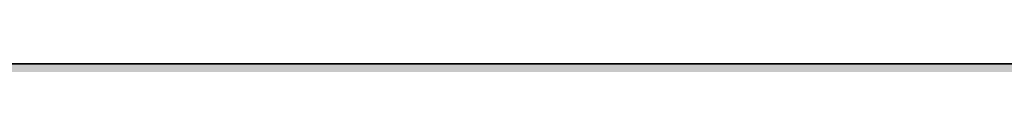
# Model space of a CAD drawing. Units: inches. Extents: x 2091 to 2899, y 967 to 2217.
# Tile 64 of 256: x 2212.2941 to 2212.646, y 1099.9191 to 1099.9191. Entities that reach past the tile are written whole.
import ezdxf

# ---------------------------------------------------------------- set-up
doc = ezdxf.new("R2010")
doc.units = ezdxf.units.IN
doc.layers.add('A-WALL-PATT', color=141, linetype='Continuous', lineweight=13, true_color=0xadddf7)
doc.layers.add('L-SITE-WALL', color=7, linetype='Continuous', lineweight=35)

msp = doc.modelspace()

# ---------------------------------------------------------------- hatches: boundary and pattern name
at = {"layer": 'A-WALL-PATT'}
h = msp.add_hatch(color=256, dxfattribs=at)
h.dxf.hatch_style = 1
h.paths.add_polyline_path([(2212.1436, 1941.41906), (2387.6436, 1941.41906), (2387.6436, 1824.41906), (2392.1436, 1824.41906), (2392.1436, 1941.41906), (2609.6436, 1941.41906), (2609.6436, 1825.91906), (2614.1436, 1825.91906), (2614.1436, 1941.41906), (2794.1436, 1941.41906), (2794.1436, 1928.76217), (2803.1436, 1928.76217), (2803.1436, 2050.91906), (2203.1436, 2050.91906), (2203.1436, 1900.75786), (2212.1436, 1900.75786)])
h.paths.add_polyline_path([(2212.1436, 1945.91906), (2212.1436, 2041.91906), (2794.1436, 2041.91906), (2794.1436, 1945.91906), (2402.24824, 1945.91906), (2401.10243, 1945.77583), (2398.70243, 1945.77583)], flags=16)
h.paths.add_polyline_path([(2230.22986, 1948.06279), (2227.34986, 1949.50279), (2225.90986, 1951.90279), (2223.98986, 1952.86279), (2223.02986, 1955.26279), (2222.06986, 1959.58279), (2222.06986, 1963.42279), (2223.02986, 1965.66279), (2223.98986, 1965.34279), (2225.58591, 1963.86075), (2226.91153, 1964.95726), (2226.94886, 1965.93879), (2227.77832, 1966.95214), (2228.19992, 1968.8787), (2230.70986, 1964.86279), (2233.58986, 1966.30279), (2233.60731, 1966.33187), (2233.77266, 1964.9382), (2234.6338, 1963.67647), (2235.02986, 1963.90279), (2236.28203, 1965.57236), (2235.98986, 1962.94279), (2237.95451, 1957.54), (2238.38986, 1957.90279), (2239.21586, 1960.30579), (2238.65457, 1966.38496), (2238.69279, 1966.43807), (2238.84058, 1967.49971), (2238.78029, 1967.68749), (2238.88054, 1967.78676), (2238.66686, 1966.25179), (2239.21586, 1960.30579), (2238.38986, 1957.90279), (2236.94986, 1956.70279), (2234.54986, 1949.98279)], flags=0)
h.paths.add_polyline_path([(2278.01197, 1948.06279), (2276.49643, 1947.87335), (2275.84983, 1947.68861), (2274.65197, 1947.10279)], flags=0)
h.paths.add_polyline_path([(2269.85197, 1955.74279), (2268.27618, 1956.62933), (2270.8673, 1956.3484), (2269.37197, 1958.14279), (2268.71496, 1959.19233), (2270.56983, 1958.72861), (2268.58073, 1961.90609), (2270.81197, 1960.89188), (2270.81197, 1963.42279), (2271.39331, 1964.77926), (2270.29176, 1966.1562), (2271.77197, 1965.66279), (2272.14139, 1966.52476), (2273.92983, 1965.92861), (2275.63039, 1968.0543), (2276.33194, 1966.72186), (2276.52043, 1966.95214), (2276.94203, 1968.8787), (2277.73429, 1967.61108), (2278.13989, 1969.46452), (2279.65912, 1967.03374), (2280.41197, 1966.78279), (2280.9493, 1967.58879), (2281.60983, 1967.36861), (2282.13327, 1968.15376), (2282.34924, 1966.33344), (2282.34985, 1966.33259), (2283.40755, 1968.09542), (2283.71263, 1965.52402), (2284.32022, 1964.63379), (2284.51181, 1964.88924), (2284.23497, 1965.70479), (2284.50047, 1967.31896), (2284.90794, 1965.41742), (2285.39631, 1966.06858), (2285.43283, 1966.29061), (2285.47334, 1966.17128), (2286.35392, 1967.34539), (2286.22201, 1966.15817), (2287.66349, 1968.08015), (2287.71397, 1968.44279), (2288.4816, 1969.01668), (2288.57399, 1968.7289), (2288.91746, 1969.06904), (2288.60683, 1966.83761), (2288.92873, 1963.35131), (2288.93497, 1963.35679), (2288.92973, 1963.34042), (2289.01528, 1962.41387), (2290.11122, 1963.87513), (2290.13283, 1963.94261), (2290.21767, 1964.01706), (2290.11122, 1963.87513), (2289.15583, 1960.89161), (2288.59404, 1959.25723), (2288.57197, 1959.10279), (2289.53197, 1960.54279), (2290.01197, 1962.46279), (2290.19184, 1962.64266), (2289.76983, 1959.68861), (2286.88983, 1957.28861), (2284.48983, 1950.56861), (2283.31466, 1950.04631), (2283.29197, 1949.98279), (2280.29006, 1948.64861), (2281.12983, 1948.64861), (2282.56983, 1948.16861), (2283.20473, 1948.06279), (2278.97197, 1948.06279), (2276.09197, 1949.50279), (2274.65197, 1951.90279), (2272.73197, 1952.86279)], flags=0)
h.paths.add_polyline_path([(2271.15887, 1958.02177), (2272.96983, 1955.84861), (2272.00983, 1960.16861), (2272.00983, 1964.00861), (2272.62443, 1965.44266), (2274.32802, 1963.86075), (2275.65365, 1964.95726), (2275.63774, 1964.53909), (2277.41223, 1966.00689), (2277.03297, 1965.15679), (2276.82992, 1964.9756), (2276.76601, 1963.29501), (2277.44964, 1962.66022), (2279.45197, 1964.86279), (2282.33197, 1966.30279), (2283.52983, 1966.88861), (2283.29451, 1966.77095), (2283.91299, 1963.8847), (2284.89925, 1964.44827), (2284.73197, 1962.94279), (2286.69662, 1957.54), (2287.13197, 1957.90279), (2287.54191, 1959.09539), (2287.7794, 1958.44231), (2285.68274, 1956.6951), (2285.8765, 1959.79534), (2284.73197, 1962.94279), (2284.89925, 1964.44827), (2283.91299, 1963.8847), (2284.22383, 1962.43412), (2283.42436, 1963.60548), (2281.60983, 1962.56861), (2281.12983, 1960.16861), (2282.08983, 1956.32861), (2283.04983, 1952.96861), (2282.56983, 1950.56861), (2280.16983, 1948.64861), (2279.88332, 1948.79187), (2278.97197, 1948.06279), (2278.97197, 1949.02279), (2278.67231, 1949.39737), (2277.28983, 1950.08861), (2275.84983, 1952.48861), (2273.92983, 1953.44861), (2272.48983, 1954.88861), (2271.92165, 1954.88861), (2271.77197, 1955.26279)], flags=0)
h.paths.add_polyline_path([(2311.99415, 1955.74279), (2312.06272, 1955.67422), (2312.0551, 1955.7085)], flags=0)
h.paths.add_polyline_path([(2331.95615, 1963.95179), (2333.39615, 1965.39179), (2331.07715, 1963.35679), (2330.9986, 1963.11152)], flags=0)
h.paths.add_polyline_path([(2310.55415, 1954.30279), (2307.03981, 1956.27994), (2310.7629, 1955.87628), (2312.47415, 1953.82279), (2313.43415, 1951.42279), (2315.35415, 1950.46279), (2316.79415, 1948.06279), (2317.46615, 1947.72679), (2319.36869, 1947.96461), (2317.75415, 1949.98279), (2317.56953, 1950.61048), (2316.79415, 1951.90279), (2314.87415, 1952.86279), (2313.91415, 1955.26279), (2311.51415, 1958.14279), (2309.37549, 1961.55917), (2311.51415, 1960.33708), (2311.51415, 1961.98279), (2310.60467, 1963.11963), (2311.72661, 1962.47853), (2312.41833, 1964.09256), (2312.25596, 1964.29552), (2313.19415, 1963.98279), (2313.91415, 1965.66279), (2314.64678, 1965.41858), (2315.35415, 1966.30279), (2316.79415, 1967.74279), (2316.15744, 1966.9469), (2317.03411, 1965.28186), (2317.2226, 1965.51214), (2317.77705, 1968.04577), (2318.47411, 1966.72186), (2318.6626, 1966.95214), (2319.0842, 1968.8787), (2321.20705, 1965.48215), (2322.16142, 1966.9137), (2322.55415, 1966.78279), (2322.78599, 1967.13056), (2322.88165, 1966.32429), (2323.31204, 1965.72174), (2323.65129, 1965.89136), (2324.3965, 1967.13338), (2324.65694, 1964.9382), (2324.97199, 1964.47661), (2325.38728, 1967.0015), (2325.94081, 1964.41835), (2327.22893, 1966.13584), (2327.16632, 1965.57236), (2328.05914, 1966.76278), (2328.22458, 1966.24749), (2329.66797, 1967.67691), (2329.66458, 1967.68749), (2329.76482, 1967.78676), (2329.55115, 1966.25179), (2330.10015, 1960.30579), (2329.33281, 1958.07347), (2329.31306, 1957.93523), (2329.63415, 1958.20279), (2330.23415, 1959.10279), (2330.71415, 1961.02279), (2331.03415, 1961.34279), (2330.71415, 1959.10279), (2329.63415, 1958.20279), (2329.27415, 1957.66279), (2327.71211, 1956.3611), (2325.43415, 1949.98279), (2324.33377, 1949.49374), (2323.99415, 1948.54279), (2319.67415, 1946.62279), (2316.79415, 1948.06279), (2315.35415, 1950.46279), (2313.43415, 1951.42279)], flags=0)
h.paths.add_polyline_path([(2321.33568, 1947.95202), (2321.11415, 1948.06279), (2321.11415, 1949.02279), (2319.19415, 1951.42279), (2316.79415, 1959.58279), (2316.66324, 1959.58279), (2315.35415, 1958.14279), (2314.39415, 1958.14279), (2313.1483, 1958.70908), (2312.95415, 1959.58279), (2312.95415, 1960.89188), (2315.83415, 1959.58279), (2316.66324, 1959.58279), (2317.31471, 1960.29941), (2315.0302, 1962.42075), (2316.35582, 1963.51726), (2316.37234, 1963.95162), (2316.4702, 1963.86075), (2317.79582, 1964.95726), (2317.75522, 1963.88969), (2319.17515, 1965.15679), (2319.49841, 1965.88137), (2321.11415, 1965.34279), (2323.23589, 1962.37236), (2325.68635, 1963.77262), (2325.54279, 1962.48058), (2325.19878, 1963.49401), (2324.47851, 1963.08243), (2324.92601, 1960.99412), (2324.07809, 1962.23647), (2322.41479, 1961.28602), (2322.07415, 1959.58279), (2323.03415, 1955.74279), (2323.99415, 1952.38279), (2323.51415, 1949.98279), (2322.14272, 1948.88565), (2322.07415, 1948.54279)], flags=0)
h.paths.add_polyline_path([(2320.20748, 1963.33746), (2320.15415, 1963.42279), (2320.39415, 1963.54279)], flags=0)
h.paths.add_polyline_path([(2353.85053, 1965.8105), (2354.03053, 1965.7505), (2354.33053, 1966.4505), (2354.33053, 1966.9305)], flags=0)
h.paths.add_polyline_path([(2359.02058, 1969.02641), (2359.09838, 1968.90193), (2359.23353, 1969.5195), (2359.23353, 1969.9995)], flags=0)
h.paths.add_polyline_path([(2358.25669, 1966.68167), (2357.9836, 1966.34803), (2358.21127, 1966.14617), (2358.41049, 1966.38957)], flags=0)
h.paths.add_polyline_path([(2357.76847, 1966.05878), (2357.7322, 1965.10497), (2357.75105, 1965.12056), (2357.76953, 1965.6065), (2357.76953, 1966.05784)], flags=0)
h.paths.add_polyline_path([(2359.11153, 1965.3045), (2359.11153, 1964.8245), (2359.84453, 1966.4675), (2359.84453, 1966.9475)], flags=0)
h.paths.add_polyline_path([(2360.22368, 1966.62145), (2360.69853, 1969.3625), (2360.69853, 1969.8425), (2360.21053, 1967.0255), (2360.21053, 1966.6425)], flags=0)
h.paths.add_polyline_path([(2363.45053, 1967.8905), (2363.45053, 1968.3705), (2362.49053, 1966.9305), (2362.65604, 1966.69878)], flags=0)
h.paths.add_polyline_path([(2364.47552, 1966.07883), (2365.85053, 1968.3705), (2365.85053, 1968.8505), (2364.42798, 1966.47958)], flags=0)
h.paths.add_polyline_path([(2366.31353, 1965.8525), (2366.36671, 1965.69583), (2366.80253, 1968.3455), (2366.80253, 1968.8255)], flags=0)
h.paths.add_polyline_path([(2367.16531, 1965.80354), (2367.29053, 1966.9305), (2367.29053, 1967.4105), (2367.1027, 1965.72007)], flags=0)
h.paths.add_polyline_path([(2370.03653, 1959.9735), (2371.01353, 1963.0245), (2371.01353, 1963.5045), (2370.03653, 1960.4535)], flags=0)
h.paths.add_polyline_path([(2371.61053, 1960.2105), (2372.57053, 1961.6505), (2372.57053, 1962.1305), (2371.80253, 1960.9785)], flags=0)
h.paths.add_polyline_path([(2350.87367, 1956.00509), (2351.93053, 1955.8905), (2354.49053, 1953.3305), (2353.85053, 1954.9305), (2351.45053, 1957.8105), (2347.93553, 1963.4255), (2347.93553, 1963.9055), (2351.45053, 1958.2905), (2353.70507, 1955.58505), (2352.89053, 1959.2505), (2352.89053, 1959.7305), (2352.89053, 1961.92479), (2356.73053, 1959.7305), (2358.45447, 1961.62684), (2354.81053, 1965.0105), (2355.03086, 1965.28591), (2358.69109, 1961.88712), (2361.53053, 1965.0105), (2364.3765, 1966.43348), (2364.52439, 1965.18691), (2365.45447, 1963.82418), (2365.88107, 1964.06795), (2365.37053, 1966.4505), (2365.37053, 1966.9305), (2366.81053, 1960.2105), (2366.81053, 1959.7305), (2366.38871, 1952.98141), (2367.77053, 1956.8505), (2368.64123, 1957.57608), (2366.81053, 1962.6105), (2366.81053, 1963.0905), (2368.77518, 1957.68771), (2369.21053, 1958.0505), (2370.00159, 1960.35187), (2369.47523, 1966.05267), (2369.51346, 1966.10578), (2369.51417, 1966.11091), (2369.47523, 1966.53267), (2369.51346, 1966.58578), (2369.61463, 1967.31259), (2369.18253, 1968.6585), (2369.18253, 1969.1385), (2369.60096, 1967.83519), (2369.7012, 1967.93447), (2369.71795, 1968.05474), (2370.14518, 1968.37414), (2369.77871, 1968.01122), (2369.7012, 1967.45447), (2370.46816, 1968.214), (2369.67494, 1967.26577), (2369.51417, 1966.11091), (2370.03653, 1960.4535), (2370.03653, 1959.9735), (2369.44176, 1958.24319), (2370.65053, 1959.2505), (2371.04582, 1962.01756), (2371.13053, 1962.1305), (2370.65053, 1958.7705), (2367.77053, 1956.3705), (2365.37053, 1949.6505), (2362.0791, 1948.18764), (2363.45053, 1947.7305), (2361.05053, 1947.7305), (2360.09053, 1947.7305), (2357.10386, 1947.35717), (2360.09053, 1948.2105), (2358.17053, 1949.1705), (2356.73053, 1951.5705), (2354.81053, 1952.5305), (2351.93053, 1955.4105)], flags=0)
h.paths.add_polyline_path([(2361.05053, 1948.6905), (2359.13053, 1951.0905), (2356.73053, 1959.2505), (2355.77053, 1959.2505), (2352.89053, 1960.55959), (2352.89053, 1961.44479), (2355.89053, 1959.7305), (2356.73053, 1959.7305), (2356.83719, 1959.36783), (2361.53053, 1964.5305), (2363.24842, 1965.38945), (2364.92531, 1963.0418), (2362.49053, 1961.6505), (2362.06386, 1959.51717), (2362.97053, 1955.8905), (2363.93053, 1952.5305), (2363.93053, 1952.0505), (2363.45053, 1949.6505), (2361.05053, 1947.7305)], flags=0)
h.paths.add_polyline_path([(2359.13053, 1951.5705), (2359.29053, 1951.3705), (2361.05053, 1954.4505), (2361.05053, 1954.9305)], flags=0)
h.paths.add_polyline_path([(2357.21953, 1966.5455), (2356.79253, 1968.8145), (2356.79253, 1969.2945), (2357.21953, 1967.0255)], flags=0)
h.paths.add_polyline_path([(2361.05053, 1954.4505), (2361.53053, 1958.7705), (2361.53053, 1959.2505), (2361.05053, 1954.9305)], flags=0)
h.paths.add_polyline_path([(2402.54829, 1948.48608), (2402.30243, 1948.41583), (2402.59043, 1948.41583)], flags=0)
h.paths.add_polyline_path([(2394.14243, 1956.09583), (2395.68505, 1954.55321), (2396.7205, 1953.97068), (2396.06243, 1955.61583), (2395.24138, 1956.6011), (2395.8789, 1956.44171), (2395.10243, 1959.93583), (2395.10243, 1963.77583), (2396.06243, 1966.01583), (2397.02243, 1965.69583), (2398.61848, 1964.21379), (2399.94411, 1965.3103), (2399.98143, 1966.29183), (2400.81089, 1967.30518), (2401.23249, 1969.23174), (2403.53795, 1965.54301), (2403.94198, 1967.38932), (2404.70243, 1967.13583), (2405.46033, 1966.07478), (2406.62243, 1966.65583), (2406.63988, 1966.68491), (2406.80523, 1965.29124), (2406.92569, 1965.11475), (2407.34243, 1964.97583), (2407.87433, 1965.77367), (2408.1691, 1964.39805), (2409.31461, 1965.9254), (2409.21746, 1965.05105), (2409.44523, 1963.13124), (2410.30637, 1961.86951), (2410.70243, 1962.09583), (2411.44227, 1963.08228), (2411.16543, 1963.89783), (2411.61643, 1966.63976), (2411.72536, 1966.79111), (2411.87315, 1967.85275), (2411.81286, 1968.04053), (2411.91311, 1968.1398), (2411.69943, 1966.60483), (2412.24843, 1960.65883), (2413.22543, 1963.70983), (2414.3779, 1964.72116), (2414.51315, 1965.69275), (2414.45286, 1965.88053), (2414.55311, 1965.9798), (2414.3779, 1964.72116), (2414.51982, 1964.8457), (2414.36536, 1964.63111), (2414.33943, 1964.44483), (2414.88843, 1958.49883), (2414.06243, 1956.09583), (2412.62243, 1954.89583), (2410.17137, 1948.03285), (2410.01672, 1948.0844), (2405.90243, 1946.25583), (2405.90243, 1947.21583), (2405.20425, 1948.08856), (2404.22243, 1948.41583), (2403.26243, 1948.41583), (2400.38243, 1949.85583), (2399.66243, 1951.05583), (2397.98243, 1952.73583), (2397.02243, 1953.21583), (2395.68505, 1954.55321), (2392.65678, 1956.25691)], flags=0)
h.paths.add_polyline_path([(2409.08565, 1964.40744), (2409.13036, 1964.27572), (2409.26243, 1964.49583)], flags=0)
h.paths.add_polyline_path([(2397.74243, 1961.61583), (2398.70243, 1963.85583), (2399.66243, 1963.53583), (2401.42656, 1965.74099), (2401.79142, 1966.5588), (2402.07143, 1965.07083), (2402.83551, 1964.39337), (2403.2624, 1964.9149), (2403.33812, 1964.77109), (2402.61552, 1963.97622), (2402.49861, 1960.90224), (2403.543, 1959.93245), (2404.4132, 1960.88968), (2404.70243, 1962.33583), (2407.91635, 1964.17235), (2409.52021, 1961.92694), (2410.98708, 1957.89304), (2411.42243, 1958.25583), (2412.04796, 1960.07562), (2412.41034, 1959.07909), (2411.67562, 1958.46682), (2411.66243, 1958.25583), (2411.62607, 1958.42553), (2409.98243, 1957.05583), (2407.58243, 1950.33583), (2403.26243, 1948.41583), (2403.26243, 1949.37583), (2401.34243, 1951.77583), (2399.41651, 1958.32398), (2397.74243, 1959.08492), (2397.74243, 1959.97012), (2397.10243, 1960.33583), (2397.74243, 1960.04492)], flags=0)
h.paths.add_polyline_path([(2405.90243, 1952.97583), (2405.95043, 1953.40783), (2406.01672, 1953.17583)], flags=0)
h.paths.add_polyline_path([(2449.81778, 1967.11401), (2449.75232, 1967.13583), (2449.7937, 1967.0779)], flags=0)
h.paths.add_polyline_path([(2451.6977, 1966.61812), (2451.74089, 1966.69012), (2451.69205, 1966.6657)], flags=0)
h.paths.add_polyline_path([(2454.34363, 1965.73757), (2455.75232, 1967.61583), (2455.99232, 1968.09583), (2454.3645, 1965.9254)], flags=0)
h.paths.add_polyline_path([(2457.54732, 1968.86383), (2457.78732, 1969.34383), (2457.05432, 1968.79583), (2457.00762, 1968.46034)], flags=0)
h.paths.add_polyline_path([(2456.92178, 1967.85666), (2456.80224, 1968.22902), (2456.723, 1967.6598)], flags=0)
h.paths.add_polyline_path([(2457.30232, 1967.37683), (2457.54232, 1967.85683), (2456.81032, 1966.83983), (2456.74052, 1966.70022), (2456.74902, 1966.60811)], flags=0)
h.paths.add_polyline_path([(2458.27532, 1963.70983), (2458.15534, 1963.33515), (2460.35432, 1965.26483), (2460.59432, 1965.74483)], flags=0)
h.paths.add_polyline_path([(2458.39232, 1962.81583), (2458.36409, 1962.61819), (2459.59232, 1964.25583), (2459.83232, 1964.73583)], flags=0)
h.paths.add_polyline_path([(2459.35232, 1962.81583), (2459.27232, 1962.49583), (2460.07232, 1963.29583), (2460.31232, 1963.77583)], flags=0)
h.paths.add_polyline_path([(2458.68032, 1960.60783), (2458.63232, 1960.41583), (2459.59232, 1961.85583), (2459.83232, 1962.33583)], flags=0)
h.paths.add_polyline_path([(2437.83817, 1956.24265), (2439.19232, 1956.09583), (2441.35232, 1953.93583), (2440.87232, 1955.13583), (2438.47232, 1958.01583), (2438.07156, 1958.65602), (2438.71232, 1958.49583), (2440.6396, 1956.18311), (2439.91232, 1959.45583), (2439.91232, 1963.29583), (2441.35232, 1966.65583), (2441.59232, 1967.13583), (2441.11232, 1966.01583), (2442.07232, 1965.69583), (2443.98899, 1968.09167), (2444.24132, 1966.75083), (2444.9168, 1966.15192), (2445.67657, 1967.08014), (2446.25532, 1969.72483), (2446.49532, 1970.20483), (2446.28238, 1969.23174), (2447.36267, 1967.50327), (2447.72032, 1969.56783), (2447.96032, 1970.04783), (2447.48548, 1967.30678), (2448.79232, 1965.21583), (2448.47232, 1964.86383), (2448.55232, 1964.73583), (2451.45205, 1966.1857), (2451.61512, 1964.81124), (2452.30792, 1963.79617), (2453.23451, 1964.32565), (2454.07232, 1960.41583), (2453.62869, 1953.31765), (2454.79232, 1956.57583), (2455.03232, 1957.05583), (2455.71884, 1957.62793), (2453.83232, 1962.81583), (2453.94097, 1963.79362), (2453.33532, 1965.57783), (2453.82432, 1968.55083), (2454.06432, 1969.03083), (2453.57532, 1966.05783), (2454.04033, 1964.68792), (2453.83232, 1962.81583), (2455.71884, 1957.62793), (2456.36721, 1958.16824), (2457.05832, 1960.17883), (2457.29832, 1960.65883), (2456.47232, 1958.25583), (2457.71773, 1959.29367), (2457.67232, 1958.97583), (2454.88995, 1956.65719), (2453.61414, 1953.08492), (2453.59232, 1952.73583), (2453.35232, 1952.25583), (2453.3596, 1952.3722), (2452.63232, 1950.33583), (2452.39232, 1949.85583), (2449.20375, 1948.43869), (2450.71232, 1947.93583), (2448.07232, 1947.93583), (2447.11232, 1947.93583), (2444.55232, 1947.61583), (2447.1996, 1948.3722), (2445.19232, 1949.37583), (2443.75232, 1951.77583), (2441.83232, 1952.73583), (2438.95232, 1955.61583)], flags=0)
h.paths.add_polyline_path([(2443.99232, 1959.93583), (2444.04032, 1959.77263), (2444.12155, 1959.86199)], flags=0)
h.paths.add_polyline_path([(2442.91232, 1959.93583), (2443.03232, 1959.93583), (2442.44566, 1960.2025)], flags=0)
h.paths.add_polyline_path([(2444.98294, 1965.01968), (2445.27932, 1965.26483), (2445.51932, 1965.74483), (2444.994, 1965.3103)], flags=0)
h.paths.add_polyline_path([(2446.13332, 1965.02983), (2446.33037, 1965.4715), (2444.97032, 1964.25783), (2444.73032, 1963.77783)], flags=0)
h.paths.add_polyline_path([(2442.79232, 1959.45583), (2443.75232, 1959.45583), (2446.15232, 1951.29583), (2446.41232, 1951.75083), (2446.39232, 1951.77583), (2448.0806, 1954.73032), (2448.55232, 1958.97583), (2441.83232, 1965.21583), (2442.15495, 1965.61911), (2448.79232, 1959.45583), (2448.31232, 1955.13583), (2448.07232, 1954.65583), (2446.41232, 1951.75083), (2448.31232, 1949.37583), (2448.31232, 1948.41583), (2450.54089, 1950.19869), (2450.95232, 1952.25583), (2449.99232, 1955.61583), (2449.03232, 1959.45583), (2449.51232, 1961.85583), (2449.75232, 1962.33583), (2449.6749, 1961.94874), (2452.99451, 1963.84565), (2453.06441, 1963.51941), (2452.88461, 1963.78285), (2449.6749, 1961.94874), (2449.27232, 1959.93583), (2450.23232, 1956.09583), (2451.19232, 1952.73583), (2450.71232, 1950.33583), (2450.47232, 1949.85583), (2448.07232, 1947.93583), (2448.07232, 1948.53583), (2445.43232, 1949.85583), (2443.99232, 1952.25583), (2442.07232, 1953.21583), (2441.11232, 1955.61583), (2440.15232, 1959.93583), (2440.15232, 1960.65583)], flags=0)
h.paths.add_polyline_path([(2456.69232, 1966.98583), (2457.60832, 1968.08083), (2457.84832, 1968.56083), (2456.93232, 1967.46583)], flags=0)
h.paths.add_polyline_path([(2489.89657, 1966.58024), (2489.94295, 1966.18935), (2490.74749, 1967.53025), (2491.31912, 1968.95116)], flags=0)
h.paths.add_polyline_path([(2473.56247, 1956.40713), (2477.13998, 1956.01926), (2476.95533, 1956.24083), (2475.10805, 1957.28011), (2476.34749, 1956.97025), (2475.1869, 1958.82422), (2476.91912, 1958.39116), (2475.41164, 1960.79927), (2477.78749, 1959.71934), (2477.78749, 1962.25025), (2477.6374, 1962.43786), (2477.82255, 1962.33206), (2478.35912, 1963.58406), (2478.35912, 1963.67116), (2477.32435, 1964.96463), (2478.71483, 1964.50114), (2479.31912, 1965.91116), (2480.27912, 1965.59116), (2481.78397, 1967.47221), (2482.11649, 1965.70525), (2482.88056, 1965.02778), (2483.20931, 1965.42941), (2483.22017, 1965.71509), (2483.07594, 1965.98902), (2483.71176, 1966.76581), (2484.13049, 1968.67925), (2484.70212, 1970.10016), (2484.48918, 1969.12707), (2486.5029, 1965.90511), (2487.38749, 1965.61025), (2488.15342, 1966.75914), (2488.71702, 1965.97011), (2489.20009, 1966.21164), (2489.33067, 1965.11099), (2490.3939, 1963.62246), (2490.66077, 1963.77496), (2490.49391, 1964.55364), (2490.92306, 1963.92484), (2491.31912, 1964.15116), (2491.33339, 1964.17018), (2491.21049, 1964.53225), (2491.28176, 1964.96554), (2491.42579, 1964.29338), (2494.07648, 1967.82763), (2494.49792, 1966.51494), (2494.59817, 1966.61422), (2494.68949, 1967.27025), (2495.10675, 1967.5822), (2495.12984, 1967.74807), (2495.06955, 1967.93585), (2495.1698, 1968.03513), (2495.03178, 1967.04363), (2495.75382, 1967.75868), (2494.98205, 1966.68644), (2494.95612, 1966.50016), (2495.47902, 1960.83685), (2495.91049, 1962.18425), (2496.48212, 1963.60516), (2496.07269, 1962.32659), (2496.7689, 1962.93754), (2496.59912, 1962.71116), (2496.11912, 1959.35116), (2496.73287, 1960.27179), (2496.98749, 1961.29025), (2497.55912, 1962.71116), (2497.07912, 1960.79116), (2496.50749, 1959.37025), (2495.54749, 1957.93025), (2492.75884, 1955.60638), (2490.83912, 1950.23116), (2490.26749, 1948.81025), (2485.94749, 1946.89025), (2483.06749, 1948.33025), (2481.62749, 1950.73025), (2479.70749, 1951.69025), (2476.82749, 1954.57025)], flags=0)
h.paths.add_polyline_path([(2485.57697, 1948.31339), (2485.55912, 1948.31116), (2485.57876, 1948.31116)], flags=0)
h.paths.add_polyline_path([(2478.64506, 1954.55116), (2478.10904, 1956.96326), (2479.31912, 1955.51116), (2480.27912, 1953.11116), (2482.19912, 1952.15116), (2483.63912, 1949.75116), (2486.51912, 1948.31116), (2486.51912, 1949.27116), (2484.73931, 1951.49593), (2484.02749, 1950.25025), (2481.62749, 1958.41025), (2482.37515, 1959.23267), (2482.19912, 1959.83116), (2483.19757, 1960.92946), (2479.70749, 1964.17025), (2480.60336, 1965.29008), (2481.87517, 1964.10911), (2482.66639, 1964.76358), (2482.61536, 1963.4218), (2482.9892, 1963.07466), (2484.00849, 1963.98425), (2484.68361, 1965.49751), (2484.58012, 1965.40516), (2485.35727, 1967.14711), (2485.12065, 1965.7812), (2486.42749, 1963.69025), (2488.14538, 1964.5492), (2489.82227, 1962.20155), (2490.74749, 1962.73025), (2491.99966, 1964.39981), (2492.07605, 1965.08726), (2492.21289, 1964.68412), (2492.48537, 1965.04743), (2492.27912, 1963.19116), (2494.24377, 1957.78837), (2494.5625, 1958.05398), (2494.93349, 1959.13325), (2495.50512, 1960.55416), (2494.67912, 1958.15116), (2494.10749, 1956.73025), (2494.5625, 1958.05398), (2493.40854, 1957.09235), (2491.70749, 1961.77025), (2491.99966, 1964.39981), (2490.74749, 1962.73025), (2487.71203, 1960.9957), (2487.47912, 1959.83116), (2488.43912, 1955.99116), (2489.39912, 1952.63116), (2488.91912, 1950.23116), (2488.57692, 1949.9574), (2488.34749, 1948.81025), (2487.65172, 1948.25363), (2487.47912, 1948.31116), (2486.51912, 1948.31116), (2483.63912, 1949.75116), (2482.19912, 1952.15116), (2480.27912, 1953.11116), (2478.83912, 1954.55116)], flags=0)
h.paths.add_polyline_path([(2526.64825, 1966.98752), (2526.51734, 1967.03116), (2526.6001, 1966.9153)], flags=0)
h.paths.add_polyline_path([(2528.47064, 1966.44666), (2528.57449, 1966.61973), (2528.45707, 1966.56102)], flags=0)
h.paths.add_polyline_path([(2534.13334, 1967.49616), (2534.15669, 1967.54285), (2534.05984, 1967.4083)], flags=0)
h.paths.add_polyline_path([(2536.16192, 1964.0506), (2535.15734, 1962.71116), (2535.10087, 1962.31587), (2536.11734, 1963.67116), (2536.42053, 1964.27754)], flags=0)
h.paths.add_polyline_path([(2535.15734, 1959.83116), (2536.11734, 1961.27116), (2536.59734, 1962.23116), (2535.25334, 1960.21516)], flags=0)
h.paths.add_polyline_path([(2513.24904, 1956.2848), (2516.22118, 1955.96256), (2514.99734, 1957.43116), (2514.19582, 1958.71154), (2515.47734, 1958.39116), (2516.93189, 1956.64571), (2516.43734, 1958.87116), (2516.43734, 1962.71116), (2516.87269, 1963.72697), (2515.34643, 1965.6348), (2517.39734, 1964.95116), (2517.87734, 1966.07116), (2518.35734, 1967.03116), (2517.87734, 1965.91116), (2518.83734, 1965.59116), (2520.48659, 1967.65272), (2520.76634, 1966.16616), (2521.53042, 1965.48869), (2521.78144, 1965.79537), (2521.80091, 1966.30727), (2521.4778, 1966.92094), (2521.24634, 1967.12616), (2521.1777, 1967.49091), (2521.4778, 1966.92094), (2522.01042, 1966.44869), (2522.25739, 1966.75042), (2522.78034, 1969.14016), (2523.26034, 1970.10016), (2523.0474, 1969.12707), (2524.67313, 1966.5259), (2526.03734, 1966.07116), (2526.79524, 1965.01011), (2527.97707, 1965.60102), (2528.14014, 1964.22657), (2528.66459, 1963.45816), (2529.38862, 1963.87189), (2529.32967, 1964.14699), (2529.48128, 1963.92484), (2529.87734, 1964.15116), (2529.98401, 1964.29338), (2529.78905, 1965.20318), (2530.0624, 1964.3979), (2532.80248, 1968.05135), (2533.14777, 1966.97585), (2533.24802, 1967.07513), (2533.33934, 1967.73116), (2533.67285, 1967.98049), (2533.72802, 1968.03513), (2533.51434, 1966.50016), (2534.02472, 1960.9725), (2534.56034, 1962.64516), (2535.04034, 1963.60516), (2534.06334, 1960.55416), (2533.23734, 1958.15116), (2534.28815, 1959.02684), (2534.19734, 1958.39116), (2531.5126, 1956.15387), (2529.39734, 1950.23116), (2528.91734, 1949.27116), (2526.44877, 1948.17402), (2527.47734, 1947.83116), (2530.35734, 1947.35116), (2524.59734, 1947.35116), (2521.71734, 1948.79116), (2520.27734, 1951.19116), (2518.35734, 1952.15116), (2515.47734, 1955.03116)], flags=0)
h.paths.add_polyline_path([(2523.93476, 1967.19031), (2523.61951, 1966.48369), (2523.7705, 1966.24211)], flags=0)
h.paths.add_polyline_path([(2518.83734, 1953.11116), (2517.87734, 1955.51116), (2516.88498, 1959.97678), (2516.91734, 1959.96207), (2516.91734, 1962.02545), (2520.75734, 1959.83116), (2522.02495, 1961.22553), (2518.35734, 1964.63116), (2519.00259, 1965.43772), (2520.43339, 1964.10911), (2521.30112, 1964.82687), (2521.24516, 1963.35533), (2525.63831, 1959.27598), (2526.03734, 1961.27116), (2529.39734, 1963.19116), (2530.64952, 1964.86073), (2530.66472, 1964.99755), (2530.69196, 1964.91731), (2531.08778, 1965.44507), (2530.94599, 1964.16894), (2530.69196, 1964.91731), (2529.39734, 1963.19116), (2526.3625, 1961.45697), (2526.03734, 1959.83116), (2526.99734, 1955.99116), (2527.95734, 1952.63116), (2527.47734, 1950.23116), (2527.13449, 1949.95687), (2526.97393, 1949.15409), (2526.69734, 1949.03116), (2524.59734, 1947.35116), (2524.59734, 1948.31116), (2524.27734, 1948.71116), (2522.19734, 1949.75116), (2520.75734, 1952.15116)], flags=0)
h.paths.add_polyline_path([(2520.27734, 1958.87116), (2520.85334, 1959.50476), (2523.15734, 1951.67116), (2524.61389, 1954.22013), (2524.59734, 1954.07116), (2522.67734, 1950.71116)], flags=0)
h.paths.add_polyline_path([(2559.37091, 1966.31116), (2559.39841, 1966.32491), (2559.40194, 1966.3453)], flags=0)
h.paths.add_polyline_path([(2549.77091, 1957.19116), (2552.65091, 1954.31116), (2552.13399, 1955.60347), (2550.61091, 1957.43116), (2547.09591, 1963.04616), (2545.77591, 1965.20616), (2549.29091, 1959.59116), (2551.69091, 1956.71116), (2550.79293, 1960.75206), (2550.73091, 1960.78025), (2550.73091, 1964.87116), (2551.69091, 1967.11116), (2552.65091, 1966.79116), (2554.24696, 1965.30911), (2555.03425, 1965.96034), (2555.58167, 1966.64461), (2555.60991, 1967.38716), (2556.43937, 1968.40051), (2556.86097, 1970.32707), (2559.37091, 1966.31116), (2560.69091, 1964.15116), (2562.40881, 1965.01011), (2561.65091, 1966.07116), (2560.33091, 1968.23116), (2561.7585, 1966.23254), (2562.34721, 1967.11561), (2562.43371, 1966.38657), (2563.1278, 1965.3696), (2563.57091, 1965.59116), (2563.58836, 1965.62024), (2563.36254, 1967.52354), (2563.72249, 1965.84379), (2565.06, 1968.07298), (2564.73286, 1965.12872), (2565.11758, 1963.33338), (2567.44462, 1966.43611), (2567.31561, 1967.83333), (2567.35384, 1967.88644), (2567.50163, 1968.94807), (2567.44134, 1969.13585), (2567.54159, 1969.23513), (2567.32791, 1967.70016), (2567.87691, 1961.75416), (2568.74669, 1964.47033), (2568.63561, 1965.67333), (2568.67384, 1965.72644), (2568.82163, 1966.78807), (2568.76134, 1966.97585), (2568.86159, 1967.07513), (2568.64791, 1965.54016), (2568.72613, 1964.69303), (2568.85391, 1964.80516), (2568.74669, 1964.47033), (2568.81724, 1963.70626), (2568.97091, 1963.91116), (2568.86607, 1963.17731), (2569.19691, 1959.59416), (2568.37091, 1957.19116), (2566.93091, 1955.99116), (2564.62027, 1949.52137), (2564.65091, 1949.51116), (2564.61662, 1949.51116), (2564.53091, 1949.27116), (2560.21091, 1947.35116), (2557.33091, 1948.79116), (2556.0452, 1950.93402), (2556.01091, 1950.95116), (2555.85662, 1951.2083), (2553.97091, 1952.15116), (2551.09091, 1955.03116), (2546.65014, 1957.52951)], flags=0)
h.paths.add_polyline_path([(2567.02579, 1959.33023), (2567.03501, 1959.30489), (2567.05091, 1959.35116)], flags=0)
h.paths.add_polyline_path([(2551.96829, 1962.51837), (2553.01091, 1964.95116), (2553.97091, 1964.63116), (2555.56696, 1963.14911), (2556.89258, 1964.24563), (2556.92991, 1965.22716), (2557.14398, 1965.48869), (2556.42007, 1966.13056), (2556.39142, 1966.10499), (2556.37991, 1966.16616), (2556.42007, 1966.13056), (2556.95191, 1966.60516), (2557.09214, 1966.91948), (2557.57087, 1966.01023), (2557.75937, 1966.24051), (2557.41791, 1964.68016), (2556.89258, 1964.24563), (2556.80709, 1961.99757), (2560.69091, 1958.39116), (2560.63553, 1957.8927), (2560.81091, 1957.19116), (2561.77091, 1953.83116), (2561.29091, 1951.43116), (2559.11042, 1949.68677), (2559.15648, 1949.62919), (2563.02652, 1951.34921), (2562.61091, 1949.27116), (2560.21091, 1947.35116), (2560.21091, 1948.31116), (2559.25091, 1949.51116), (2558.89091, 1949.51116), (2558.89091, 1949.96116), (2558.29091, 1950.71116), (2558.0537, 1951.51767), (2556.97091, 1952.87116), (2555.06788, 1959.34146), (2552.05091, 1961.06545), (2552.05091, 1962.47116)], flags=0)
h.paths.add_polyline_path([(2588.33005, 1958.39116), (2588.61025, 1958.11096), (2588.55336, 1958.36695)], flags=0)
h.paths.add_polyline_path([(2594.74545, 1950.49309), (2593.95753, 1953.17202), (2593.13005, 1954.55116), (2591.21005, 1955.51116), (2590.25005, 1957.91116), (2588.30903, 1960.24038), (2586.17731, 1961.20935), (2587.85005, 1960.79116), (2587.25342, 1961.74425), (2588.44131, 1961.06545), (2588.44131, 1962.65553), (2588.42168, 1962.66535), (2588.44131, 1962.71116), (2586.91404, 1964.62026), (2588.87709, 1963.72796), (2589.29005, 1964.69154), (2589.29005, 1966.07116), (2590.25005, 1968.31116), (2591.21005, 1967.99116), (2592.8061, 1966.50911), (2594.13172, 1967.60563), (2594.16905, 1968.58716), (2594.99851, 1969.60051), (2595.4201, 1971.52707), (2597.93005, 1967.51116), (2600.81005, 1968.95116), (2600.8275, 1968.98024), (2600.99285, 1967.58657), (2601.85399, 1966.32484), (2602.10714, 1966.4695), (2602.23635, 1967.25507), (2602.35672, 1966.69338), (2603.50222, 1968.22073), (2603.21005, 1965.59116), (2605.1747, 1960.18837), (2605.50689, 1960.4652), (2605.02602, 1965.67333), (2605.06425, 1965.72644), (2605.21203, 1966.78807), (2605.15174, 1966.97585), (2605.25199, 1967.07513), (2605.34331, 1967.73116), (2605.9529, 1968.1869), (2605.87475, 1969.03333), (2605.91298, 1969.08644), (2606.06077, 1970.14807), (2606.00048, 1970.33585), (2606.10073, 1970.43513), (2605.88705, 1968.90016), (2606.43605, 1962.95416), (2605.61005, 1960.55116), (2605.99704, 1960.87365), (2606.56431, 1962.64516), (2608.24149, 1964.11694), (2608.01005, 1963.19116), (2607.05005, 1961.75116), (2606.63149, 1961.40236), (2606.20131, 1958.39116), (2603.32131, 1955.99116), (2600.92131, 1949.27116), (2596.60131, 1947.35116), (2593.72131, 1948.79116), (2592.85731, 1950.23116), (2592.65005, 1950.23116)], flags=0)
h.paths.add_polyline_path([(2596.60131, 1947.35116), (2596.60131, 1948.31116), (2594.68131, 1950.71116), (2596.15495, 1953.29003), (2595.53005, 1954.07116), (2593.19923, 1961.99596), (2592.65134, 1962.50471), (2591.78015, 1963.00253), (2593.28299, 1964.24563), (2593.32031, 1965.22716), (2594.14977, 1966.24051), (2594.57137, 1968.16707), (2596.18265, 1965.58902), (2596.95127, 1966.43451), (2598.04131, 1966.07116), (2598.79921, 1965.01011), (2599.96131, 1965.59116), (2599.97876, 1965.62024), (2600.14411, 1964.22657), (2601.00526, 1962.96484), (2601.40131, 1963.19116), (2602.65349, 1964.86073), (2602.36131, 1962.23116), (2603.79275, 1958.29472), (2601.97764, 1953.21243), (2601.94621, 1952.70945), (2599.46876, 1951.60836), (2599.00131, 1949.27116)], flags=0)
h.paths.add_polyline_path([(2597.56131, 1958.87116), (2597.67097, 1959.41942), (2597.59505, 1958.7362)], flags=0)
h.paths.add_polyline_path([(2623.6663, 1961.25438), (2625.51916, 1960.79116), (2624.96554, 1961.67553), (2627.19916, 1960.66025), (2627.19916, 1961.15116), (2626.95916, 1962.23116), (2626.95916, 1963.49116), (2625.58232, 1965.21221), (2626.95916, 1964.42545), (2626.95916, 1965.83116), (2626.86916, 1965.86116), (2627.91916, 1968.31116), (2628.87916, 1967.99116), (2630.47521, 1966.50911), (2631.80084, 1967.60563), (2631.83816, 1968.58716), (2632.66762, 1969.60051), (2633.08922, 1971.52707), (2635.59916, 1967.51116), (2638.47916, 1968.95116), (2638.49661, 1968.98024), (2638.66196, 1967.58657), (2639.17627, 1966.83301), (2639.78022, 1967.83958), (2640.02583, 1966.69338), (2641.17134, 1968.22073), (2640.87916, 1965.59116), (2641.11426, 1964.94463), (2641.41134, 1965.34073), (2641.3081, 1964.41159), (2642.84381, 1960.18837), (2643.27916, 1960.55116), (2644.08474, 1962.89474), (2643.78387, 1966.15333), (2643.80683, 1966.18524), (2643.60068, 1968.41805), (2643.52281, 1968.66058), (2643.72988, 1970.14807), (2643.66959, 1970.33585), (2643.76984, 1970.43513), (2643.55616, 1968.90016), (2643.60068, 1968.41805), (2643.90959, 1967.45585), (2644.00984, 1967.55513), (2643.81174, 1966.13208), (2644.10516, 1962.95416), (2644.23877, 1961.35084), (2644.71916, 1961.75116), (2645.03285, 1962.2217), (2645.32216, 1963.12516), (2646.07642, 1963.78705), (2645.03285, 1962.2217), (2644.34516, 1960.07416), (2643.51916, 1957.67116), (2642.07916, 1956.47116), (2639.71961, 1949.86442), (2639.87553, 1949.83843), (2635.35916, 1947.83116), (2632.47916, 1949.27116), (2631.03916, 1951.67116), (2629.11916, 1952.63116), (2628.15916, 1955.03116), (2625.75916, 1957.91116)], flags=0)
h.paths.add_polyline_path([(2627.81631, 1956.57402), (2627.37371, 1958.56571), (2626.37631, 1959.76259), (2627.19916, 1959.35116), (2627.37371, 1958.56571), (2627.91916, 1957.91116), (2628.87916, 1955.51116), (2630.79916, 1954.55116), (2632.23916, 1952.15116), (2633.31502, 1951.61323), (2631.03916, 1959.35116), (2631.49783, 1959.85569), (2630.79916, 1962.23116), (2631.44987, 1962.94694), (2630.71521, 1963.62911), (2632.04084, 1964.72563), (2632.07816, 1965.70716), (2632.29224, 1965.96869), (2631.70534, 1966.48907), (2633.13644, 1967.76614), (2633.32922, 1968.64707), (2634.67472, 1966.49427), (2635.20847, 1967.08139), (2636.79916, 1966.55116), (2637.6764, 1967.86702), (2638.99395, 1966.02246), (2639.70534, 1966.42898), (2641.11916, 1959.83116), (2640.93007, 1956.80571), (2639.43916, 1952.63116), (2638.22746, 1952.09262), (2637.75916, 1949.75116), (2635.35916, 1947.83116), (2635.35916, 1948.79116), (2633.43916, 1951.19116), (2633.31502, 1951.61323), (2632.23916, 1952.15116), (2630.79916, 1954.55116), (2628.87916, 1955.51116)], flags=0)
h.paths.add_polyline_path([(2637.75916, 1953.83116), (2637.27916, 1955.51116), (2636.31916, 1959.35116), (2636.79916, 1961.75116), (2639.23395, 1963.14246), (2637.55706, 1965.49011), (2638.73889, 1966.08102), (2638.90196, 1964.70657), (2639.7631, 1963.44484), (2636.79916, 1961.75116), (2636.5325, 1960.41783), (2637.03916, 1958.39116), (2637.99916, 1955.03116)], flags=0)
h.paths.add_polyline_path([(2668.56741, 1951.43116), (2667.60741, 1953.83116), (2665.20741, 1956.71116), (2662.2939, 1961.36531), (2665.44741, 1959.59116), (2666.64741, 1958.39116), (2666.64741, 1959.97516), (2666.05832, 1960.68207), (2666.64741, 1960.34545), (2666.64741, 1961.99116), (2666.70009, 1962.11409), (2666.40741, 1963.43116), (2666.40741, 1967.27116), (2667.36741, 1969.51116), (2668.32741, 1969.19116), (2669.92346, 1967.70911), (2671.24908, 1968.80563), (2671.28641, 1969.78716), (2672.11587, 1970.80051), (2672.53746, 1972.72707), (2675.04741, 1968.71116), (2677.92741, 1970.15116), (2677.94486, 1970.18024), (2678.11021, 1968.78657), (2678.97135, 1967.52484), (2679.36741, 1967.75116), (2680.61958, 1969.42073), (2680.32741, 1966.79116), (2682.29206, 1961.38837), (2682.72741, 1961.75116), (2683.35831, 1963.58657), (2683.23211, 1964.95333), (2683.27034, 1965.00644), (2683.39322, 1965.88914), (2683.35997, 1966.24921), (2683.35784, 1966.25585), (2683.35923, 1966.25723), (2682.99211, 1970.23333), (2683.03034, 1970.28644), (2683.17812, 1971.34807), (2683.11784, 1971.53585), (2683.21808, 1971.63513), (2683.00441, 1970.10016), (2683.35923, 1966.25723), (2683.45808, 1966.35513), (2683.39322, 1965.88914), (2683.41391, 1965.66502), (2684.42381, 1966.87227), (2683.55341, 1964.15416), (2683.35831, 1963.58657), (2683.79341, 1958.87416), (2682.96741, 1956.47116), (2681.52741, 1955.27116), (2680.10923, 1951.30025), (2680.08493, 1950.91157), (2679.97685, 1950.92959), (2679.12741, 1948.55116), (2674.80741, 1946.63116), (2671.92741, 1948.07116), (2670.48741, 1950.47116)], flags=0)
h.paths.add_polyline_path([(2671.93568, 1953.22702), (2671.68741, 1953.35116), (2670.24741, 1955.75116), (2668.32741, 1956.71116), (2667.35674, 1959.13783), (2669.52741, 1958.15116), (2670.48741, 1958.15116), (2671.47941, 1959.24236), (2670.6844, 1961.94538), (2668.8896, 1963.61198), (2667.30741, 1964.33116), (2668.56741, 1963.91116), (2668.83094, 1964.24057), (2670.24741, 1963.43116), (2672.42214, 1965.82337), (2672.77746, 1967.44707), (2673.23407, 1966.71649), (2674.41192, 1968.01212), (2673.98056, 1965.52211), (2675.28741, 1963.43116), (2675.55407, 1963.56449), (2675.93241, 1965.45616), (2676.24741, 1965.35116), (2677.0053, 1964.29011), (2678.16741, 1964.87116), (2679.60741, 1967.27116), (2680.32741, 1963.91116), (2680.30655, 1963.57748), (2680.34724, 1963.45761), (2680.85958, 1964.14073), (2680.56741, 1961.51116), (2681.10362, 1960.03657), (2678.88741, 1953.83116), (2677.09248, 1953.03341), (2677.68741, 1950.95116), (2677.20741, 1948.55116), (2674.80741, 1946.63116), (2674.80741, 1947.59116), (2672.88741, 1949.99116)], flags=0)
h.paths.add_polyline_path([(2673.98455, 1951.91116), (2674.56741, 1952.93116), (2674.56741, 1951.91116), (2676.96741, 1953.83116), (2677.44741, 1956.23116), (2676.48741, 1959.59116), (2676.24741, 1960.55116), (2679.72959, 1962.54098), (2680.05927, 1961.00248), (2679.21135, 1962.24484), (2676.24741, 1960.55116), (2676.48741, 1959.59116), (2677.44741, 1956.23116), (2676.96741, 1953.83116), (2674.56741, 1951.91116)], flags=0)
h.paths.add_polyline_path([(2707.47928, 1952.81465), (2706.51928, 1955.21465), (2705.55928, 1959.53465), (2705.55928, 1963.37465), (2706.51928, 1965.61465), (2707.47928, 1965.29465), (2709.07533, 1963.81261), (2710.40096, 1964.90912), (2710.43828, 1965.89065), (2711.26774, 1966.904), (2711.68934, 1968.83056), (2714.19928, 1964.81465), (2717.07928, 1966.25465), (2717.09673, 1966.28373), (2717.26208, 1964.89006), (2718.12322, 1963.62833), (2718.51928, 1963.85465), (2719.77146, 1965.52422), (2719.47928, 1962.89465), (2721.44393, 1957.49186), (2721.87928, 1957.85465), (2722.70528, 1960.25765), (2722.14399, 1966.33682), (2722.18221, 1966.38993), (2722.33, 1967.45157), (2722.26971, 1967.63934), (2722.36996, 1967.73862), (2722.15628, 1966.20365), (2722.70528, 1960.25765), (2721.87928, 1957.85465), (2720.43928, 1956.65465), (2718.03928, 1949.93465), (2713.71928, 1948.01465), (2710.83928, 1949.45465), (2709.39928, 1951.85465)], flags=0)
h.paths.add_polyline_path([(2749.30123, 1952.81465), (2748.34123, 1955.21465), (2747.38123, 1959.53465), (2747.38123, 1963.37465), (2748.34123, 1965.61465), (2749.30123, 1965.29465), (2750.89728, 1963.81261), (2752.2229, 1964.90912), (2752.26023, 1965.89065), (2753.08969, 1966.904), (2753.51129, 1968.83056), (2756.02123, 1964.81465), (2758.90123, 1966.25465), (2758.91868, 1966.28373), (2759.08403, 1964.89006), (2759.94517, 1963.62833), (2760.34123, 1963.85465), (2761.5934, 1965.52422), (2761.30123, 1962.89465), (2763.26588, 1957.49186), (2763.70123, 1957.85465), (2764.52723, 1960.25765), (2763.96594, 1966.33682), (2764.00416, 1966.38993), (2764.15195, 1967.45157), (2764.09166, 1967.63934), (2764.19191, 1967.73862), (2763.97823, 1966.20365), (2764.52723, 1960.25765), (2763.70123, 1957.85465), (2762.26123, 1956.65465), (2759.86123, 1949.93465), (2755.54123, 1948.01465), (2752.66123, 1949.45465), (2751.22123, 1951.85465)], flags=0)
h.paths.add_polyline_path([(2212.1436, 1819.93451), (2203.1436, 1819.93451), (2203.1436, 1739.97955), (2212.1436, 1739.97955), (2212.1436, 1780.91906), (2392.1436, 1780.91906), (2392.1436, 1783.91906), (2212.1436, 1783.91906)])
h.paths.add_polyline_path([(2803.1436, 1847.93882), (2794.1436, 1847.93882), (2794.1436, 1785.41906), (2609.6436, 1785.41906), (2493.87561, 1785.41906), (2493.87561, 1780.91906), (2609.6436, 1780.91906), (2794.1436, 1780.91906), (2794.1436, 1696.91906), (2609.37561, 1696.91906), (2609.37561, 1742.91906), (2604.87561, 1742.91906), (2604.87561, 1644.41906), (2609.37561, 1644.41906), (2609.37561, 1692.41906), (2794.1436, 1692.41906), (2794.1436, 1668.16474), (2803.1436, 1668.16474)])
h.paths.add_polyline_path([(2392.1436, 1740.41906), (2387.6436, 1740.41906), (2387.6436, 1629.41906), (2212.1436, 1629.41906), (2212.1436, 1659.1562), (2203.1436, 1659.1562), (2203.1436, 1494.08944), (2212.1436, 1494.08944), (2212.1436, 1627.91906), (2392.1436, 1627.91906)])
h.paths.add_polyline_path([(2457.87561, 1780.91906), (2453.37561, 1780.91906), (2453.37561, 1644.41906), (2568.87561, 1644.41906), (2568.87561, 1648.91906), (2457.87561, 1648.91906)])
h.paths.add_polyline_path([(2545.1436, 1591.91906), (2540.6436, 1591.91906), (2540.6436, 1567.91906), (2468.6436, 1567.91906), (2468.6436, 1627.91906), (2509.1436, 1627.91906), (2509.1436, 1632.41906), (2464.1436, 1632.41906), (2464.1436, 1563.41906), (2545.1436, 1563.41906)])
h.paths.add_polyline_path([(2268.6436, 1555.91906), (2212.1436, 1555.91906), (2212.1436, 1551.41906), (2268.6436, 1551.41906)], flags=17)
h.paths.add_polyline_path([(2212.1436, 1413.26609), (2203.1436, 1413.26609), (2203.1436, 1233.0704), (2212.1436, 1233.0704)])
h.paths.add_polyline_path([(2267.6436, 1351.91906), (2212.1436, 1351.91906), (2212.1436, 1347.41906), (2267.6436, 1347.41906)], flags=17)
h.paths.add_polyline_path([(2456.6436, 1489.41906), (2452.1436, 1489.41906), (2452.1436, 1351.91906), (2312.6436, 1351.91906), (2312.6436, 1347.41906), (2456.6436, 1347.41906)])
h.paths.add_polyline_path([(2472.37017, 1455.41906), (2467.87017, 1455.41906), (2467.87017, 1347.41906), (2472.37017, 1347.41906)])
h.paths.add_polyline_path([(2794.1436, 1351.91906), (2543.37017, 1351.91906), (2543.37017, 1347.41906), (2794.1436, 1347.41906)], flags=17)
h.paths.add_polyline_path([(2312.6436, 1347.41906), (2308.1436, 1347.41906), (2308.1436, 1302.16179), (2308.34197, 1302.16433), (2308.1436, 1298.16925), (2308.1436, 1275.41906), (2212.1436, 1275.41906), (2212.1436, 1270.91906), (2312.6436, 1270.91906)], flags=17)
h.paths.add_polyline_path([(2212.1436, 1152.24706), (2203.1436, 1152.24706), (2203.1436, 1090.91906), (2803.1436, 1090.91906), (2803.1436, 1392.71355), (2794.1436, 1392.71355), (2794.1436, 1143.41906), (2548.03245, 1143.41906), (2548.03245, 1138.91906), (2794.1436, 1138.91906), (2794.1436, 1099.91906), (2212.1436, 1099.91906)])
h.paths.add_polyline_path([(2471.53245, 1266.32853, 0.031658), (2467.03245, 1269.94579), (2467.03245, 1143.41906), (2471.53245, 1143.41906), (2471.53245, 1148.81906)], flags=17)
h.paths.add_polyline_path([(2803.1436, 1587.34139), (2794.1436, 1587.34139), (2794.1436, 1473.5369), (2803.1436, 1473.5369)])
h.paths.add_polyline_path([(2794.1436, 1536.41906), (2651.1436, 1536.41906), (2651.1436, 1531.91906), (2794.1436, 1531.91906)])
h.paths.add_polyline_path([(2614.1436, 1620.41906), (2609.6436, 1620.41906), (2609.6436, 1536.41906), (2614.1436, 1536.41906)])
h.paths.add_polyline_path([(2271.08273, 1964.31724), (2776.85297, 1964.31724), (2776.85297, 2037.16962), (2271.08273, 2037.16962)], flags=8)
h.paths.add_polyline_path([(2380.64929, 1536.82414), (2461.04081, 1536.82414), (2461.04081, 1554.65259), (2380.64929, 1554.65259)], flags=9)
h.paths.add_polyline_path([(2203.65504, 1608.81531), (2316.11844, 1608.81531), (2316.11844, 1621.91836), (2203.65504, 1621.91836)], flags=24)
h.paths.add_polyline_path([(2212.67726, 1313.5041), (2282.59152, 1313.5041), (2282.59152, 1322.74524), (2212.67726, 1322.74524)], flags=24)
h.paths.add_polyline_path([(2457.11198, 1114.77857), (2558.48158, 1114.77857), (2558.48158, 1142.21968), (2457.11198, 1142.21968)], flags=25)
h.paths.add_polyline_path([(2473.44234, 1273.01007), (2604.64123, 1273.01007), (2604.64123, 1318.34693), (2473.44234, 1318.34693)], flags=25)
h.paths.add_polyline_path([(2638.8763, 1626.97743), (2684.25037, 1627.97674), (2684.03848, 1637.59749), (2638.66442, 1636.59819)], flags=9)
h.paths.add_polyline_path([(2537.59055, 1453.79345), (2628.38955, 1453.79345), (2628.38955, 1475.34481), (2537.59055, 1475.34481)], flags=9)
h.paths.add_polyline_path([(2504.13764, 1714.6324), (2554.64719, 1714.6324), (2554.64719, 1730.23771), (2504.13764, 1730.23771)], flags=25)
h.paths.add_polyline_path([(2487.50118, 1575.65187), (2535.09712, 1575.65187), (2535.09712, 1598.37765), (2487.50118, 1598.37765)], flags=25)
h.paths.add_polyline_path([(2709.0994, 1735.71028), (2740.0166, 1735.71028), (2740.0166, 1749.93764), (2709.0994, 1749.93764)], flags=25)
h.paths.add_polyline_path([(2442.43842, 1792.17166), (2564.72884, 1792.17166), (2564.72884, 1842.00016), (2442.43842, 1842.00016)], flags=9)
h.paths.add_polyline_path([(2655.8158, 1809.64408), (2789.52014, 1806.6938), (2790.08498, 1832.29164), (2656.38064, 1835.24192)], flags=25)
h.paths.add_polyline_path([(2234.8427, 1797.72014), (2368.59285, 1794.76885), (2369.16072, 1820.50413), (2235.41056, 1823.45542)], flags=9)
h.paths.add_polyline_path([(2245.13847, 1644.00633), (2398.42773, 1640.6239), (2398.99484, 1666.32482), (2245.70557, 1669.70725)], flags=9)
h.paths.add_polyline_path([(2306.14285, 1431.16852), (2413.76831, 1428.79369), (2414.33315, 1454.39153), (2306.70768, 1456.76636)], flags=9)
h.paths.add_polyline_path([(2306.83458, 1458.23314), (2393.38048, 1456.32345), (2393.93281, 1481.35436), (2307.38691, 1483.26405)], flags=9)

# ---------------------------------------------------------------- linework, layer by layer
at = {"layer": 'L-SITE-WALL'}
msp.add_line((2794.1436, 1099.91906), (2212.1436, 1099.91906), dxfattribs=at)

doc.saveas('drawing.dxf')
